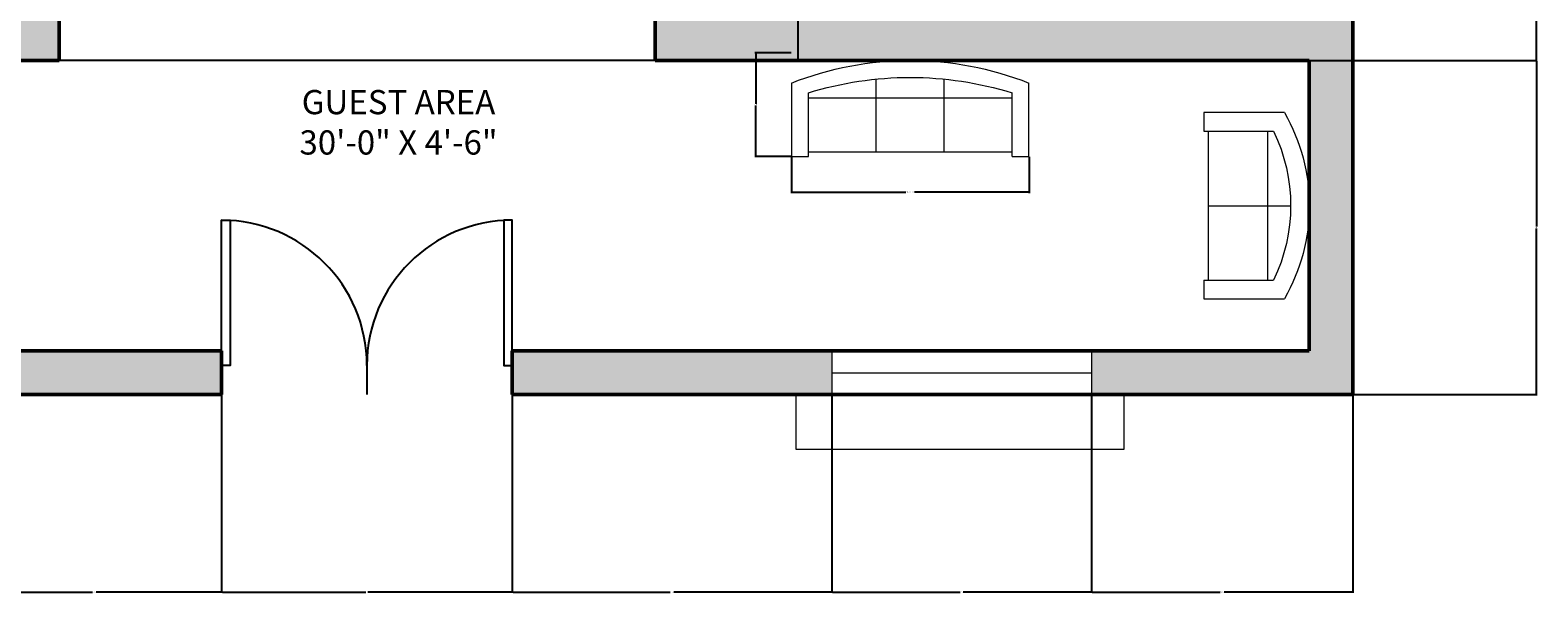
# Model space of a CAD drawing. Units: inches. Extents: x 2710 to 3197, y 524 to 1147.
# Tile 2 of 6: x 2885 to 3197, y 524 to 640. Entities that reach past the tile are written whole.
import ezdxf

# ---------------------------------------------------------------- set-up
doc = ezdxf.new("R2010")
doc.units = ezdxf.units.IN
for name, color, linetype, lineweight in [('A-ANNO-DIMS', 2, 'Continuous', 18), ('A-AREA-IDEN', 7, 'Continuous', 25), ('A-DOOR', 3, 'Continuous', 25), ('A-FLOR-STRS', 7, 'Continuous', 25), ('A-FURN', 8, 'Continuous', 18), ('A-GLAZ', 4, 'Continuous', 18), ('A-WALL', 7, 'Continuous', 50), ('A-WALL-PATT', 74, 'Continuous', 13)]:
    doc.layers.add(name, color=color, linetype=linetype, lineweight=lineweight)
doc.styles.get("Standard").update_dxf_attribs({"font": 'arial.ttf'})
doc.dimstyles.get("Standard").update_dxf_attribs({"dimtxt": 0.18, "dimasz": 0.18, "dimexe": 0.18, "dimexo": 0.0625, "dimgap": 0.09, "dimtad": 0, "dimtih": 1, "dimtoh": 1, "dimdec": 4, "dimzin": 0, "dimdsep": 46, "dimtxsty": 'Standard', "dimcen": 0.09, "dimadec": 0, "dimazin": 0, "dimtfac": 1, "dimtdec": 4, "dimtofl": 0, "dimtmove": 0, "dimatfit": 3, "dimfxl": 1, "dimtolj": 1, "dimtzin": 0, "dimarcsym": 0})

# ---------------------------------------------------------------- blocks, each defined once
blk = doc.blocks.new('*U11')
for p, q in [((0, 0), (0, -6)), ((30, 0), (30, -6))]:
    blk.add_line(p, q)
blk.add_lwpolyline([(0, 0), (0, 30), (1.75, 30), (1.75, 0)], close=True)
blk.add_arc((0, 0), 30, 0, 90)
blk = doc.blocks.new('*U12')
for p, q in [((-30, 0), (-30, -6)), ((0, 0), (0, -6))]:
    blk.add_line(p, q)
blk.add_lwpolyline([(0, 0), (0, 30), (-1.75, 30), (-1.75, 0)], close=True)
blk.add_arc((0, 0), 30, 90, 180)
blk = doc.blocks.new('Sofa - Roundback 7 ft.')
for p, q in [((-12.00002, -32.4421), (-12.00003, -6.5971)), ((11.99997, -32.4421), (11.99998, -6.5971)), ((-36.000027, -34), (-36.000027, -11.4696)), ((-35.999844, -13.3819), (35.9998, -13.3819)), ((35.99998, -34), (35.99998, -11.4696)), ((-36.000027, -32.4421), (35.99998, -32.4421))]:
    blk.add_line(p, q)
for points in [[(-36.000027, -34), (-42.000027, -34), (-42.000027, -8)], [(41.99998, -8), (41.99998, -34), (35.99998, -34)]]:
    blk.add_lwpolyline(points)
for centre, radius, start, end in [((0, -114.25), 114.25, 68.43141, 111.5686), ((-0.00001, -127.1968), 121.1968, 72.72033, 107.2797)]:
    blk.add_arc(centre, radius, start, end)
blk = doc.blocks.new('Sofa - Roundback Loveseat 5 ft.')
for p, q in [((0, -32.44198), (0, -5.99998)), ((-24, -33.99998), (-24, -11.46958)), ((-23.9998, -13.38178), (23.99986, -13.38178)), ((24.00004, -33.99998), (24.00004, -11.46958)), ((-24, -32.44198), (24.00004, -32.44198))]:
    blk.add_line(p, q)
for points in [[(-24, -33.99998), (-30, -33.99998), (-30, -7.99998)], [(30.00004, -7.99998), (30.00004, -33.99998), (24.00004, -33.99998)]]:
    blk.add_lwpolyline(points)
for centre, radius, start, end in [((0, -60.24998), 60.24998, 60.13715, 119.8628), ((0, -61.38438), 55.38444, 64.32083, 115.6792)]:
    blk.add_arc(centre, radius, start, end)
blk = doc.blocks.new('*D30')
at = {"layer": 'A-ANNO-DIMS', "color": 0, "lineweight": -2, "transparency": 16777216}
for p, q in [((3042.46, 614.09), (3042.46, 606.61)), ((3091.51, 614.09), (3091.51, 606.61)), ((3042.64, 606.79), (3066.08, 606.79)), ((3091.33, 606.79), (3067.89, 606.79))]:
    blk.add_line(p, q, dxfattribs=at)
at = {"layer": 'A-ANNO-DIMS', "color": 0, "transparency": 16777216}
for points in [[(3042.64, 606.82), (3042.64, 606.76), (3042.46, 606.79)], [(3091.33, 606.82), (3091.33, 606.76), (3091.51, 606.79)]]:
    blk.add_solid(points, dxfattribs=at)
at = {"layer": 'Defpoints', "color": 0, "transparency": 16777216}
for p in [(3042.46, 614.15), (3091.51, 614.15), (3042.46, 606.79)]:
    blk.add_point(p, dxfattribs=at)
at = {"layer": 'A-ANNO-DIMS', "color": 0, "transparency": 16777216, "insert": (3066.99, 606.79), "char_height": 0.18, "attachment_point": 5}
blk.add_mtext('\\A1;SOFA 49 TYP.', dxfattribs=at)
blk = doc.blocks.new('*D31')
at = {"layer": 'A-ANNO-DIMS', "color": 0, "lineweight": -2, "transparency": 16777216}
for p, q in [((3042.4, 635.56), (3034.93, 635.56)), ((3035.11, 635.38), (3035.11, 625.04)), ((3035.11, 614.33), (3035.11, 624.67)), ((3042.4, 614.15), (3034.93, 614.15))]:
    blk.add_line(p, q, dxfattribs=at)
at = {"layer": 'A-ANNO-DIMS', "color": 0, "transparency": 16777216}
for points in [[(3035.08, 635.38), (3035.14, 635.38), (3035.11, 635.56)], [(3035.08, 614.33), (3035.14, 614.33), (3035.11, 614.15)]]:
    blk.add_solid(points, dxfattribs=at)
at = {"layer": 'Defpoints', "color": 0, "transparency": 16777216}
for p in [(3035.11, 635.56), (3042.46, 635.56), (3042.46, 614.15)]:
    blk.add_point(p, dxfattribs=at)
at = {"layer": 'A-ANNO-DIMS', "color": 0, "transparency": 16777216, "insert": (3035.11, 624.85), "char_height": 0.18, "attachment_point": 5}
blk.add_mtext('\\A1;21 TYP.', dxfattribs=at)
blk = doc.blocks.new('*D45')
at = {"layer": 'A-ANNO-DIMS', "color": 0, "lineweight": -2, "transparency": 16777216}
for p, q in [((2872.37, 564.94), (2872.37, 524.03)), ((2924.85, 564.94), (2924.85, 524.03)), ((2872.55, 524.21), (2898.22, 524.21)), ((2924.67, 524.21), (2899, 524.21))]:
    blk.add_line(p, q, dxfattribs=at)
at = {"layer": 'A-ANNO-DIMS', "color": 0, "transparency": 16777216}
for points in [[(2872.55, 524.24), (2872.55, 524.18), (2872.37, 524.21)], [(2924.67, 524.24), (2924.67, 524.18), (2924.85, 524.21)]]:
    blk.add_solid(points, dxfattribs=at)
at = {"layer": 'Defpoints', "color": 0, "transparency": 16777216}
for p in [(2872.37, 565), (2924.85, 565), (2924.85, 524.21)]:
    blk.add_point(p, dxfattribs=at)
at = {"layer": 'A-ANNO-DIMS', "color": 0, "transparency": 16777216, "insert": (2898.61, 524.21), "char_height": 0.18, "attachment_point": 5}
blk.add_mtext('\\A1;52.48', dxfattribs=at)
blk = doc.blocks.new('*D46')
at = {"layer": 'A-ANNO-DIMS', "color": 0, "lineweight": -2, "transparency": 16777216}
for p, q in [((2924.85, 564.94), (2924.85, 524.03)), ((2984.85, 564.94), (2984.85, 524.03)), ((2925.03, 524.21), (2954.63, 524.21)), ((2984.67, 524.21), (2955.07, 524.21))]:
    blk.add_line(p, q, dxfattribs=at)
at = {"layer": 'A-ANNO-DIMS', "color": 0, "transparency": 16777216}
for points in [[(2925.03, 524.24), (2925.03, 524.18), (2924.85, 524.21)], [(2984.67, 524.24), (2984.67, 524.18), (2984.85, 524.21)]]:
    blk.add_solid(points, dxfattribs=at)
at = {"layer": 'Defpoints', "color": 0, "transparency": 16777216}
for p in [(2924.85, 565), (2984.85, 565), (2984.85, 524.21)]:
    blk.add_point(p, dxfattribs=at)
at = {"layer": 'A-ANNO-DIMS', "color": 0, "transparency": 16777216, "insert": (2954.85, 524.21), "char_height": 0.18, "attachment_point": 5}
blk.add_mtext('\\A1;60', dxfattribs=at)
blk = doc.blocks.new('*D47')
at = {"layer": 'A-ANNO-DIMS', "color": 0, "lineweight": -2, "transparency": 16777216}
for p, q in [((2984.85, 564.94), (2984.85, 524.03)), ((3050.79, 564.94), (3050.79, 524.03)), ((2985.03, 524.21), (3017.43, 524.21)), ((3050.61, 524.21), (3018.21, 524.21))]:
    blk.add_line(p, q, dxfattribs=at)
at = {"layer": 'A-ANNO-DIMS', "color": 0, "transparency": 16777216}
for points in [[(2985.03, 524.24), (2985.03, 524.18), (2984.85, 524.21)], [(3050.61, 524.24), (3050.61, 524.18), (3050.79, 524.21)]]:
    blk.add_solid(points, dxfattribs=at)
at = {"layer": 'Defpoints', "color": 0, "transparency": 16777216}
for p in [(2984.85, 565), (3050.79, 565), (3050.79, 524.21)]:
    blk.add_point(p, dxfattribs=at)
at = {"layer": 'A-ANNO-DIMS', "color": 0, "transparency": 16777216, "insert": (3017.82, 524.21), "char_height": 0.18, "attachment_point": 5}
blk.add_mtext('\\A1;65.94', dxfattribs=at)
blk = doc.blocks.new('*D48')
at = {"layer": 'A-ANNO-DIMS', "color": 0, "lineweight": -2, "transparency": 16777216}
for p, q in [((3050.79, 564.94), (3050.79, 524.03)), ((3104.39, 564.94), (3104.39, 524.03)), ((3050.97, 524.21), (3077.27, 524.21)), ((3104.21, 524.21), (3077.92, 524.21))]:
    blk.add_line(p, q, dxfattribs=at)
at = {"layer": 'A-ANNO-DIMS', "color": 0, "transparency": 16777216}
for points in [[(3050.97, 524.24), (3050.97, 524.18), (3050.79, 524.21)], [(3104.21, 524.24), (3104.21, 524.18), (3104.39, 524.21)]]:
    blk.add_solid(points, dxfattribs=at)
at = {"layer": 'Defpoints', "color": 0, "transparency": 16777216}
for p in [(3050.79, 565), (3104.39, 565), (3104.39, 524.21)]:
    blk.add_point(p, dxfattribs=at)
at = {"layer": 'A-ANNO-DIMS', "color": 0, "transparency": 16777216, "insert": (3077.59, 524.21), "char_height": 0.18, "attachment_point": 5}
blk.add_mtext('\\A1;53.6', dxfattribs=at)
blk = doc.blocks.new('*D49')
at = {"layer": 'A-ANNO-DIMS', "color": 0, "lineweight": -2, "transparency": 16777216}
for p, q in [((3104.39, 564.94), (3104.39, 524.03)), ((3158.35, 564.94), (3158.35, 524.03)), ((3104.57, 524.21), (3130.98, 524.21)), ((3158.17, 524.21), (3131.76, 524.21))]:
    blk.add_line(p, q, dxfattribs=at)
at = {"layer": 'A-ANNO-DIMS', "color": 0, "transparency": 16777216}
for points in [[(3104.57, 524.24), (3104.57, 524.18), (3104.39, 524.21)], [(3158.17, 524.24), (3158.17, 524.18), (3158.35, 524.21)]]:
    blk.add_solid(points, dxfattribs=at)
at = {"layer": 'Defpoints', "color": 0, "transparency": 16777216}
for p in [(3104.39, 565), (3158.35, 565), (3158.35, 524.21)]:
    blk.add_point(p, dxfattribs=at)
at = {"layer": 'A-ANNO-DIMS', "color": 0, "transparency": 16777216, "insert": (3131.37, 524.21), "char_height": 0.18, "attachment_point": 5}
blk.add_mtext('\\A1;53.96', dxfattribs=at)
blk = doc.blocks.new('*D57')
at = {"layer": 'A-ANNO-DIMS', "color": 0, "lineweight": -2, "transparency": 16777216}
for p, q in [((3149.41, 634), (3196.41, 634)), ((3196.23, 633.82), (3196.23, 599.68)), ((3196.23, 565.18), (3196.23, 599.32)), ((3158.41, 565), (3196.41, 565))]:
    blk.add_line(p, q, dxfattribs=at)
at = {"layer": 'A-ANNO-DIMS', "color": 0, "transparency": 16777216}
for points in [[(3196.2, 633.82), (3196.26, 633.82), (3196.23, 634)], [(3196.2, 565.18), (3196.26, 565.18), (3196.23, 565)]]:
    blk.add_solid(points, dxfattribs=at)
at = {"layer": 'Defpoints', "color": 0, "transparency": 16777216}
for p in [(3149.35, 634), (3196.23, 634), (3158.35, 565)]:
    blk.add_point(p, dxfattribs=at)
at = {"layer": 'A-ANNO-DIMS', "color": 0, "transparency": 16777216, "insert": (3196.23, 599.5), "char_height": 0.18, "attachment_point": 5}
blk.add_mtext('\\A1;69', dxfattribs=at)
blk = doc.blocks.new('*D58')
at = {"layer": 'A-ANNO-DIMS', "color": 0, "lineweight": -2, "transparency": 16777216}
for p, q in [((3158.41, 685.53), (3196.41, 685.53)), ((3196.23, 685.35), (3196.23, 659.95)), ((3196.23, 634.18), (3196.23, 659.59)), ((3149.41, 634), (3196.41, 634))]:
    blk.add_line(p, q, dxfattribs=at)
at = {"layer": 'A-ANNO-DIMS', "color": 0, "transparency": 16777216}
for points in [[(3196.2, 685.35), (3196.26, 685.35), (3196.23, 685.53)], [(3196.2, 634.18), (3196.26, 634.18), (3196.23, 634)]]:
    blk.add_solid(points, dxfattribs=at)
at = {"layer": 'Defpoints', "color": 0, "transparency": 16777216}
for p in [(3158.35, 685.53), (3196.23, 685.53), (3149.35, 634)]:
    blk.add_point(p, dxfattribs=at)
at = {"layer": 'A-ANNO-DIMS', "color": 0, "transparency": 16777216, "insert": (3196.23, 659.77), "char_height": 0.18, "attachment_point": 5}
blk.add_mtext('\\A1;51.53', dxfattribs=at)
blk = doc.blocks.new('*D71')
at = {"layer": 'A-ANNO-DIMS', "color": 0, "lineweight": -2, "transparency": 16777216}
for p, q in [((3014.41, 670), (3044.03, 670)), ((3043.85, 669.82), (3043.85, 652.18)), ((3043.85, 634.18), (3043.85, 651.82)), ((3014.41, 634), (3044.03, 634))]:
    blk.add_line(p, q, dxfattribs=at)
at = {"layer": 'A-ANNO-DIMS', "color": 0, "transparency": 16777216}
for points in [[(3043.82, 669.82), (3043.88, 669.82), (3043.85, 670)], [(3043.82, 634.18), (3043.88, 634.18), (3043.85, 634)]]:
    blk.add_solid(points, dxfattribs=at)
at = {"layer": 'Defpoints', "color": 0, "transparency": 16777216}
for p in [(3014.35, 670), (3014.35, 634), (3043.85, 634)]:
    blk.add_point(p, dxfattribs=at)
at = {"layer": 'A-ANNO-DIMS', "color": 0, "transparency": 16777216, "insert": (3043.85, 652), "char_height": 0.18, "attachment_point": 5}
blk.add_mtext('\\A1;36', dxfattribs=at)

msp = doc.modelspace()

# ---------------------------------------------------------------- hatches: boundary and pattern name
at = {"layer": 'A-WALL-PATT'}
h = msp.add_hatch(color=256, dxfattribs=at)
h.dxf.hatch_style = 1
h.paths.add_polyline_path([(2898.3484, 1096.0017), (2898.3484, 967.0017), (2948.3484, 967.0017), (2948.3484, 787.0017), (2957.3484, 787.0017), (2957.3484, 793.0017), (2957.3484, 833.0017), (2957.3484, 967.0017), (3007.3484, 967.0017), (3007.3484, 973.0017), (3007.3484, 1009.0017), (3007.3484, 1096.0017), (3149.3484, 1096.0017), (3149.3484, 1084.4601), (3158.3484, 1084.4601), (3158.3484, 1105.0017), (2991.781, 1105.0017), (2991.781, 1096.0017), (2998.3484, 1096.0017), (2998.3484, 976.0017), (2957.3484, 976.0017), (2957.3484, 1003.0017), (2966.3484, 1003.0017), (2966.3484, 1012.0017), (2957.3484, 1012.0017), (2957.3484, 1096.0017), (2963.4487, 1096.0017), (2963.4487, 1105.0017), (2940.703, 1105.0017), (2940.703, 1096.0017), (2948.3484, 1096.0017), (2948.3484, 1012.0017), (2939.3484, 1012.0017), (2939.3484, 1003.0017), (2948.3484, 1003.0017), (2948.3484, 976.0017), (2907.3484, 976.0017), (2907.3484, 1096.0017), (2916.9598, 1096.0017), (2916.9598, 1105.0017), (2857.03, 1105.0017), (2857.03, 1096.0017)])
h.paths.add_polyline_path([(2789.8274, 1096.0017), (2789.8274, 1105.0017), (2747.3484, 1105.0017), (2747.3484, 943.327), (2756.3484, 943.327), (2756.3484, 967.0017), (2828.3484, 967.0017), (2828.3484, 909.0017), (2837.3484, 909.0017), (2837.3484, 967.0017), (2862.3484, 967.0017), (2862.3484, 973.0017), (2862.3484, 976.0017), (2756.3484, 976.0017), (2756.3484, 1096.0017)])
h.paths.add_polyline_path([(2828.3484, 868.0017), (2828.3484, 830.0017), (2837.3484, 830.0017), (2837.3484, 877.0017), (2756.3484, 877.0017), (2756.3484, 904.8338), (2747.3484, 904.8338), (2747.3484, 858.8554), (2756.3484, 858.8554), (2756.3484, 868.0017)])
h.paths.add_polyline_path([(2747.3484, 742.5572), (2756.3484, 742.5572), (2756.3484, 787.0017), (2849.3484, 787.0017), (2849.3484, 796.0017), (2837.3484, 796.0017), (2837.3484, 802.0017), (2831.3484, 802.0017), (2828.3484, 802.0017), (2828.3484, 796.0017), (2756.3484, 796.0017), (2756.3484, 819.3052), (2747.3484, 819.3052)])
h.paths.add_polyline_path([(2756.3484, 643.0017), (2756.3484, 672.4477), (2747.3484, 672.4477), (2747.3484, 565.0017), (2825.5051, 565.0017), (2825.5051, 574.0017), (2756.3484, 574.0017), (2756.3484, 634.0017), (2891.3484, 634.0017), (2891.3484, 787.0017), (2908.3484, 787.0017), (2908.3484, 793.0017), (2908.3484, 796.0017), (2891.3484, 796.0017), (2885.3484, 796.0017), (2885.3484, 790.0017), (2885.3484, 754.0017), (2885.3484, 643.0017)])
h.paths.add_polyline_path([(2924.8484, 565.0017), (2924.8484, 571.0017), (2924.8484, 574.0017), (2872.3715, 574.0017), (2872.3715, 565.0017)])
h.paths.add_polyline_path([(2984.8484, 574.0017), (2984.8484, 571.0017), (2984.8484, 565.0017), (3050.793, 565.0017), (3050.793, 574.0017)])
h.paths.add_polyline_path([(3158.3484, 565.0017), (3158.3484, 685.5326), (3149.3484, 685.5326), (3149.3484, 675.4542), (3149.3484, 643.0017), (3020.3484, 643.0017), (3020.3484, 796.0017), (3014.3484, 796.0017), (2997.3484, 796.0017), (2997.3484, 787.0017), (3014.3484, 787.0017), (3014.3484, 634.0017), (3149.3484, 634.0017), (3149.3484, 574.0017), (3104.3903, 574.0017), (3104.3903, 565.0017)])
h.paths.add_polyline_path([(3149.3484, 787.0017), (3149.3484, 746.9465), (3158.3484, 746.9465), (3158.3484, 820.3805), (3149.3484, 820.3805), (3149.3484, 796.0017), (3077.3484, 796.0017), (3077.3484, 802.0017), (3074.3484, 802.0017), (3068.3484, 802.0017), (3068.3484, 796.0017), (3056.3484, 796.0017), (3056.3484, 790.0017), (3056.3484, 787.0017)])
h.paths.add_polyline_path([(3158.3484, 905.224), (3149.3484, 905.224), (3149.3484, 877.0017), (3068.3484, 877.0017), (3068.3484, 838.0017), (3074.3484, 838.0017), (3077.3484, 838.0017), (3077.3484, 868.0017), (3149.3484, 868.0017), (3149.3484, 852.3022), (3158.3484, 852.3022)], flags=17)
h.paths.add_polyline_path([(3099.2867, 814.3126), (3142.0289, 814.3126), (3142.0289, 832.97), (3099.2867, 832.97)], flags=25)
h.paths.add_polyline_path([(2981.8144, 832.8032), (3033.605, 832.8032), (3033.605, 851.4605), (2981.8144, 851.4605)], flags=25)

# ---------------------------------------------------------------- linework, layer by layer
at = {"layer": 'A-FLOR-STRS'}
msp.add_line((3014.3484, 634.0017), (2891.3484, 634.0017), dxfattribs=at)
at = {"layer": 'A-GLAZ'}
for p, q in [((3050.793, 574.0017), (3050.793, 565.0017)), ((3104.3903, 574.0017), (3104.3903, 565.0017)), ((3050.793, 569.5017), (3104.3903, 569.5017)), ((3043.3703, 565.0017), (3043.3703, 553.7139)), ((3111.13, 553.7139), (3111.13, 565.0017)), ((3043.3703, 553.7139), (3111.13, 553.7139))]:
    msp.add_line(p, q, dxfattribs=at)
at = {"layer": 'A-WALL'}
for p, q in [((3158.3484, 565.0017), (3158.3484, 1105.0017)), ((2891.3484, 787.0017), (2891.3484, 634.0017)), ((3014.3484, 634.0017), (3014.3484, 787.0017)), ((2891.3484, 634.0017), (2756.3484, 634.0017)), ((3149.3484, 634.0017), (3014.3484, 634.0017)), ((3149.3484, 574.0017), (3149.3484, 634.0017)), ((2756.3484, 574.0017), (2924.8484, 574.0017)), ((2924.8484, 565.0017), (2924.8484, 574.0017)), ((2984.8484, 565.0017), (2984.8484, 574.0017)), ((2984.8484, 574.0017), (3149.3484, 574.0017)), ((2747.3484, 565.0017), (2924.8484, 565.0017)), ((2984.8484, 565.0017), (3158.3484, 565.0017))]:
    msp.add_line(p, q, dxfattribs=at)

# ---------------------------------------------------------------- block references
at = {"layer": 'A-DOOR'}
for name, p in [('*U11', (2924.8484, 571.0017)), ('*U12', (2984.8484, 571.0017))]:
    msp.add_blockref(name, p, dxfattribs=at)
at = {"layer": 'A-FURN', "xscale": -0.5838396323201516, "yscale": 0.5838396323201516, "zscale": 0.5838396323201516}
msp.add_blockref('Sofa - Roundback 7 ft.', (3066.9859, 634.0017), dxfattribs=at)
at = {"layer": 'A-FURN', "xscale": -0.640698906201209, "yscale": 0.640698906201209, "zscale": 0.640698906201209, "rotation": 270}
msp.add_blockref('Sofa - Roundback Loveseat 5 ft.', (3149.3484, 604.0017), dxfattribs=at)

# ---------------------------------------------------------------- texts
at = {"layer": 'A-AREA-IDEN', "insert": (2932.55, 627.8909), "char_height": 5, "attachment_point": 1}
msp.add_mtext_dynamic_manual_height_columns('\\pxqc;GUEST AREA\\P30\'-0" X 4\'-6"', width=57.655828, gutter_width=12.5, heights=[0], dxfattribs=at)

# ---------------------------------------------------------------- dimensions: what is measured, and where the dimension line sits
at = {"layer": 'A-ANNO-DIMS'}
for base, p1, p2, angle, override, picture, middle in [((3196.2275, 685.5326), (3149.3484, 634.0017), (3158.3484, 685.5326), 90, {"dimdec": 2, "dimlfac": 1, "dimrnd": 0, "dimzin": 0, "dimdsep": 46, "dimlunit": 2}, '*D58', (3196.2275, 659.7671)), ((3043.8484, 634.0017), (3014.3484, 670.0017), (3014.3484, 634.0017), 270, {"dimdec": 0, "dimlfac": 1, "dimrnd": 0, "dimzin": 0, "dimdsep": 46, "dimlunit": 2}, '*D71', (3043.8484, 652.0017)), ((3196.2275, 634.0017), (3158.3484, 565.0017), (3149.3484, 634.0017), 90, {"dimdec": 0, "dimlfac": 1, "dimrnd": 0, "dimzin": 0, "dimdsep": 46, "dimlunit": 2}, '*D57', (3196.2275, 599.5017))]:
    dim = msp.add_linear_dim(base=base, p1=p1, p2=p2, angle=angle, dimstyle='Standard', override=override, dxfattribs=at)
    dim.commit()
    dim.dimension.update_dxf_attribs({"geometry": picture, "text_midpoint": middle})
for base, p1, p2, angle, text, picture, middle in [((3035.1082, 635.5586), (3042.4646, 614.1511), (3042.4646, 635.5586), 90, '<> TYP.', '*D31', (3035.1082, 624.8548)), ((3042.4646, 606.7947), (3091.5071, 614.1511), (3042.4646, 614.1511), 180, 'SOFA <> TYP.', '*D30', (3066.9859, 606.7947))]:
    dim = msp.add_linear_dim(base=base, p1=p1, p2=p2, angle=angle, text=text, dimstyle='Standard', override={"dimdec": 0, "dimlfac": 1, "dimrnd": 0, "dimzin": 0, "dimdsep": 46, "dimlunit": 2}, dxfattribs=at)
    dim.commit()
    dim.dimension.update_dxf_attribs({"geometry": picture, "text_midpoint": middle})
for base, p1, p2, override, picture, middle in [((2924.8484, 524.2139), (2872.3715, 565.0017), (2924.8484, 565.0017), {"dimdec": 2, "dimlfac": 1, "dimrnd": 0, "dimzin": 0, "dimdsep": 46, "dimlunit": 2}, '*D45', (2898.61, 524.2139)), ((2984.8484, 524.2139), (2924.8484, 565.0017), (2984.8484, 565.0017), {"dimdec": 0, "dimlfac": 1, "dimrnd": 0, "dimzin": 0, "dimdsep": 46, "dimlunit": 2}, '*D46', (2954.8484, 524.2139)), ((3050.793, 524.2139), (2984.8484, 565.0017), (3050.793, 565.0017), {"dimdec": 2, "dimlfac": 1, "dimrnd": 0, "dimzin": 0, "dimdsep": 46, "dimlunit": 2}, '*D47', (3017.8207, 524.2139)), ((3104.3903, 524.2139), (3050.793, 565.0017), (3104.3903, 565.0017), {"dimdec": 1, "dimlfac": 1, "dimrnd": 0, "dimzin": 0, "dimdsep": 46, "dimlunit": 2}, '*D48', (3077.5917, 524.2139)), ((3158.3484, 524.2139), (3104.3903, 565.0017), (3158.3484, 565.0017), {"dimdec": 2, "dimlfac": 1, "dimrnd": 0, "dimzin": 0, "dimdsep": 46, "dimlunit": 2}, '*D49', (3131.3694, 524.2139))]:
    dim = msp.add_linear_dim(base=base, p1=p1, p2=p2, dimstyle='Standard', override=override, dxfattribs=at)
    dim.commit()
    dim.dimension.update_dxf_attribs({"geometry": picture, "text_midpoint": middle})

doc.saveas('drawing.dxf')
